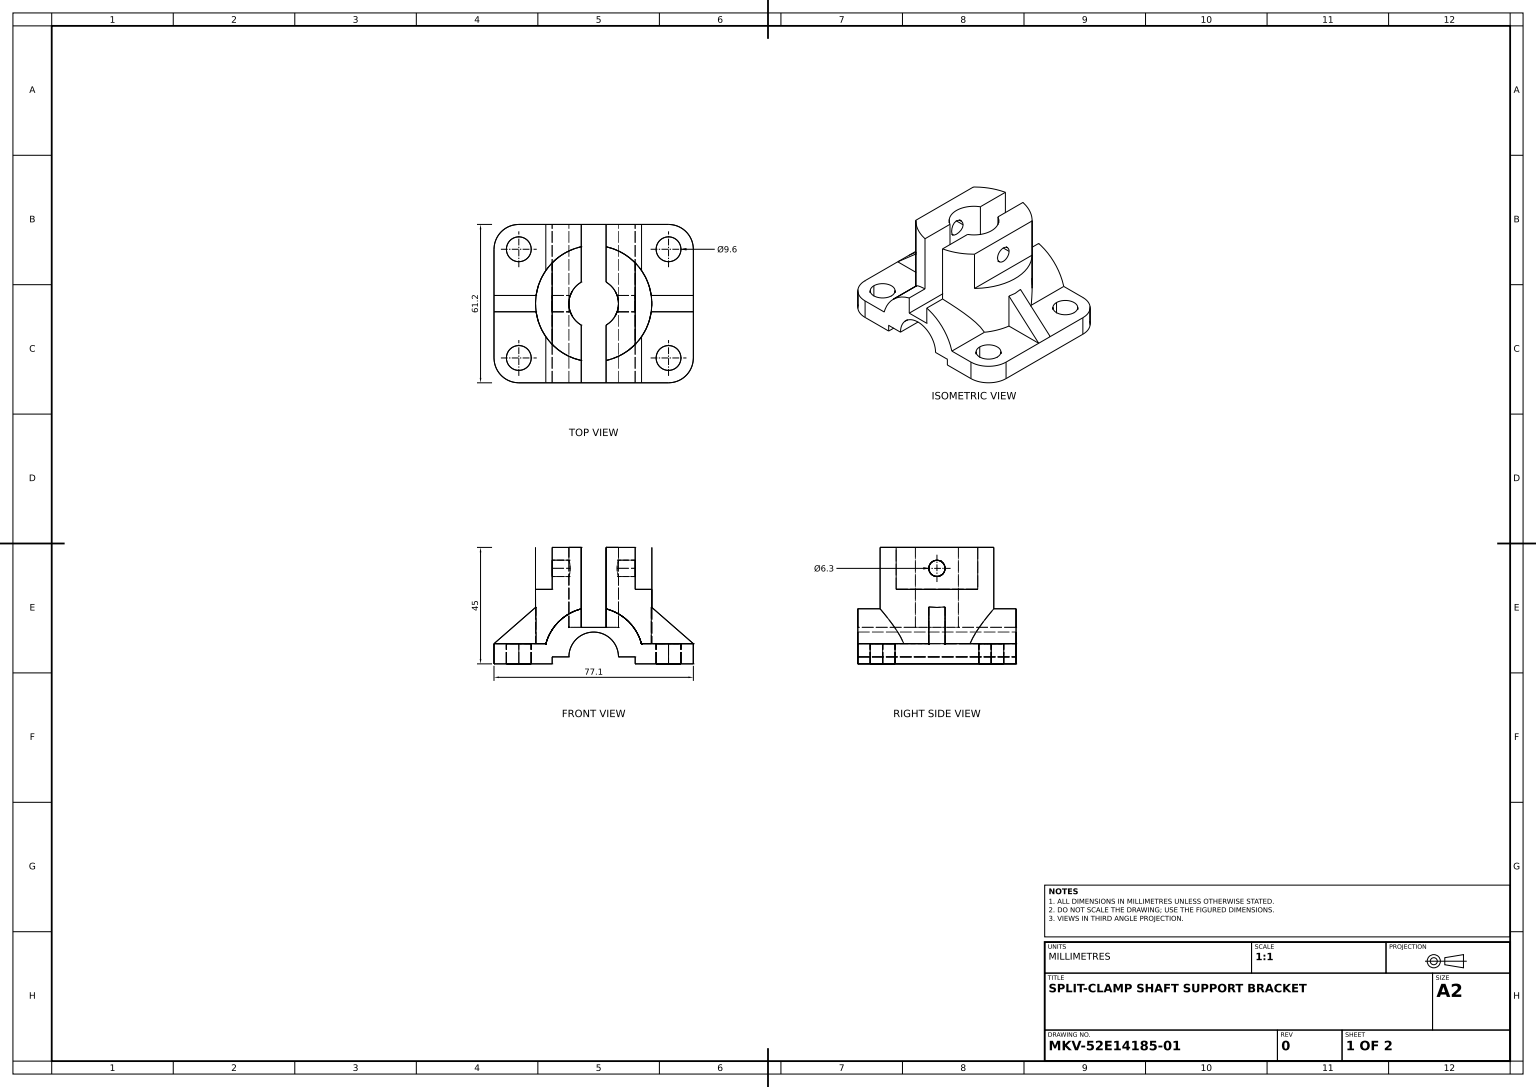
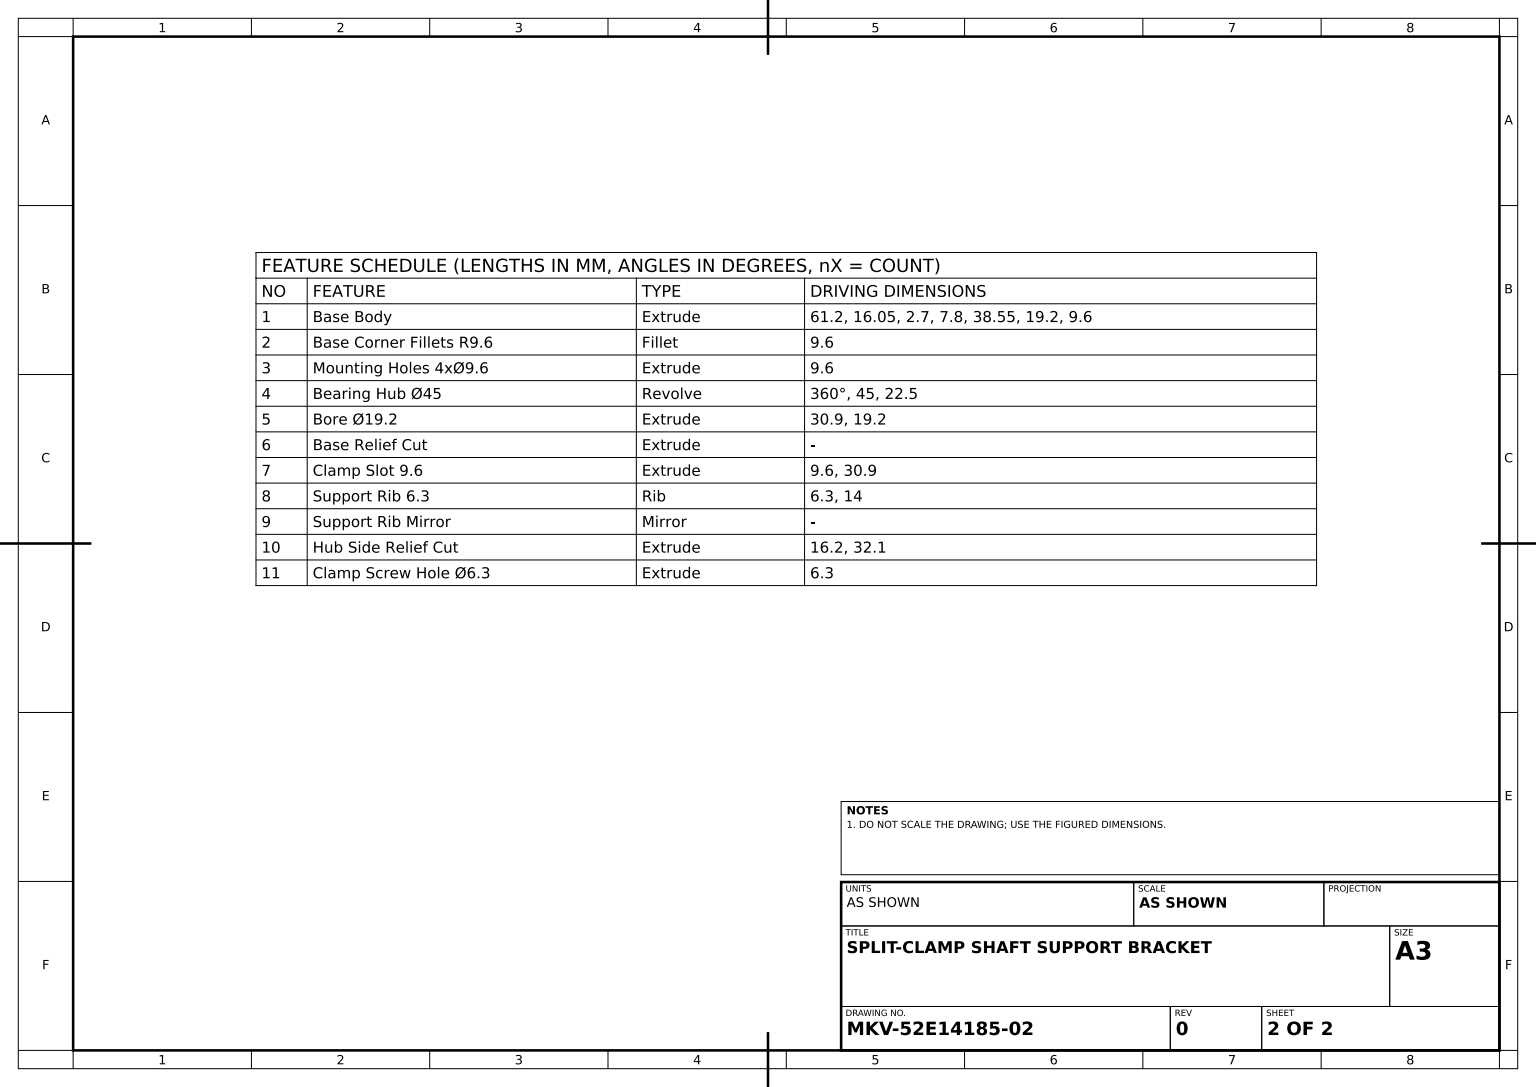
SolidWorks part; units mm, degrees
material "Plain Carbon Steel"
ref_plane "Front Plane" through (0, 0, 0) normal (0, 0, 1) x (1, 0, 0)
ref_plane "Top Plane" through (0, 0, 0) normal (0, 1, 0) x (1, 0, 0)
ref_plane "Right Plane" through (0, 0, 0) normal (1, 0, 0) x (0, 0, -1)
sketch "Base Body Profile Sketch" plane through (0, 0, 0) normal (0, 0, 1) x (1, 0, 0)
  line L0 (-19.2, 0) -> (68.6175, 0) construction
  line L1 (9.6, 0) -> (16.05, 0)
  line L2 (16.05, 0) -> (16.05, -2.7)
  line L3 (16.05, -2.7) -> (38.55, -2.7)
  line L4 (38.55, -2.7) -> (38.55, 5.1)
  line L5 (38.55, 5.1) -> (18.5103, 5.1)
  line L6 (0, 0) -> (0, 28.5519) construction
  line L7 (-38.55, 5.1) -> (-18.5103, 5.1)
  line L8 (-38.55, -2.7) -> (-38.55, 5.1)
  line L9 (-16.05, -2.7) -> (-38.55, -2.7)
  line L10 (-16.05, 0) -> (-16.05, -2.7)
  line L11 (-9.6, 0) -> (-16.05, 0)
  arc A1 (9.6, 0) -> (-9.6, 0) centre (0, 0) ccw
  arc A2 (18.5103, 5.1) -> (-18.5103, 5.1) centre (0, 0) ccw
  dimension "D1" = 16.05
  dimension "D2" = 9.6
  dimension "D6" = 19.2
  dimension "D3" = 2.7
  dimension "D4" = 7.8
  dimension "D5" = 38.55
extrude "Base Body" add sketch "Base Body Profile Sketch" along normal mid plane 61.2
fillet "Base Corner Fillets R9.6" radius 9.6 4 edges at (38.55, 1.2, -30.6) (-38.55, 1.2, -30.6) (38.55, 1.2, 30.6) (-38.55, 1.2, 30.6)
sketch "Mounting Holes Sketch" plane through (0, 5.1, 0) normal (0, 1, 0) x (1, 0, 0)
  circle A0 centre (-28.95, 21) radius 4.8
  arc A1 (-28.95, 30.6) -> (-38.55, 21) centre (-28.95, 21) ccw construction
  circle A2 centre (-28.95, -21) radius 4.8
  circle A3 centre (28.95, -21) radius 4.8
  circle A4 centre (28.95, 21) radius 4.8
  arc A5 (-38.55, -21) -> (-28.95, -30.6) centre (-28.95, -21) ccw construction
  arc A6 (28.95, -30.6) -> (38.55, -21) centre (28.95, -21) ccw construction
  arc A7 (38.55, 21) -> (28.95, 30.6) centre (28.95, 21) ccw construction
  dimension "D1" = 9.6
extrude "Mounting Holes 4xØ9.6" cut sketch "Mounting Holes Sketch" against normal up to next
sketch "Bearing Hub Profile Sketch" plane through (0, 0, 0) normal (0, 0, 1) x (1, 0, 0)
  line L0 (0, 5.1) -> (0, 42.3)
  line L1 (0, 42.3) -> (22.5, 42.3)
  line L2 (22.5, 42.3) -> (22.5, 5.1)
  line L3 (28.95, 5.1) -> (18.5103, 5.1) construction
  line L5 (16.05, -2.7) -> (28.95, -2.7) construction
  line L6 (22.5, 5.1) -> (0, 5.1)
  dimension "D1" = 22.5
  dimension "D2" = 45
revolve "Bearing Hub Ø45" add sketch "Bearing Hub Profile Sketch" angle 360 about L0
sketch "Bore Sketch" plane through (0, 42.3, 0) normal (0, 1, 0) x (1, 0, 0)
  circle A0 centre (0, 0) radius 9.6
  dimension "D1" = 19.2
extrude "Bore Ø19.2" cut sketch "Bore Sketch" against normal blind 30.9
sketch "Base Relief Sketch" plane through (0, 0, 30.6) normal (0, 0, 1) x (1, 0, 0)
  line L0 (-9.6, 0) -> (9.6, 0)
  arc A0 (9.6, 0) -> (-9.6, 0) centre (0, 0) ccw construction
  arc A1 (9.6, 0) -> (-9.6, 0) centre (0, 0) ccw
extrude "Base Relief Cut" cut sketch "Base Relief Sketch" against normal through all
sketch "Clamp Slot Sketch" plane through (0, 0, 30.6) normal (0, 0, 1) x (1, 0, 0)
  line L0 (9.6, 42.3) -> (-9.6, 42.3) construction
  line L1 (-4.8, 11.4) -> (4.8, 11.4)
  line L2 (-4.8, 11.4) -> (-4.8, 42.3)
  line L3 (-4.8, 42.3) -> (4.8, 42.3)
  line L4 (4.8, 11.4) -> (4.8, 42.3)
  point P6 (0, 11.4)
  point P8 (0, 42.3)
  dimension "D1" = 9.6
  dimension "D2" = 30.9
extrude "Clamp Slot 9.6" cut sketch "Clamp Slot Sketch" against normal through all
sketch "Support Rib Sketch" plane through (0, 0, 0) normal (0, 0, 1) x (1, 0, 0)
  line L0 (-22.5, 19.1) -> (-38.55, 5.1)
  line L1 (-22.5, 42.3) -> (-22.5, 5.1) construction
  dimension "D1" = 14
rib "Support Rib 6.3" sketch "Support Rib Sketch" sketch "Support Rib Sketch" thickness 6.3 extrusion direction parallel to sketch draft on no parameters "D1"=6.3
mirror "Support Rib Mirror" about plane through (0, 0, 0) normal (1, 0, 0) of "Support Rib 6.3"
sketch "Hub Side Relief Sketch" plane through (0, 0, 0) normal (0, 0, 1) x (1, 0, 0)
  line L0 (0, 0) -> (0, 49.9151) construction
  line L1 (-22.5, 42.3) -> (-16.05, 42.3)
  line L2 (-22.5, 42.3) -> (-22.5, 26.1)
  line L3 (-22.5, 26.1) -> (-16.05, 26.1)
  line L4 (-16.05, 42.3) -> (-16.05, 26.1)
  line L5 (22.5, 26.1) -> (16.05, 26.1)
  line L6 (16.05, 42.3) -> (16.05, 26.1)
  line L7 (22.5, 42.3) -> (22.5, 26.1)
  line L8 (22.5, 42.3) -> (16.05, 42.3)
  dimension "D1" = 32.1
  dimension "D2" = 16.2
extrude "Hub Side Relief Cut" cut sketch "Hub Side Relief Sketch" against normal through all both and the other way through all
sketch "Clamp Screw Hole Sketch" plane through (0, 0, 0) normal (1, 0, 0) x (0, 0, -1)
  line L0 (15.7686, 26.1) -> (15.7686, 42.3) construction
  circle A0 centre (0, 34.2) radius 3.15
  point P4 (15.7686, 34.2)
  dimension "D1" = 6.3
extrude "Clamp Screw Hole Ø6.3" cut sketch "Clamp Screw Hole Sketch" against normal through all both and the other way through all
